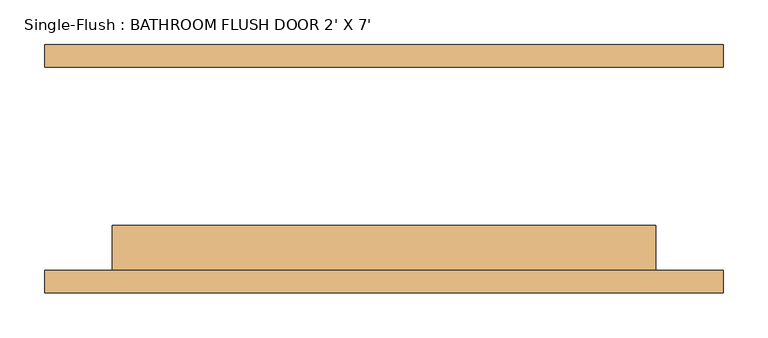
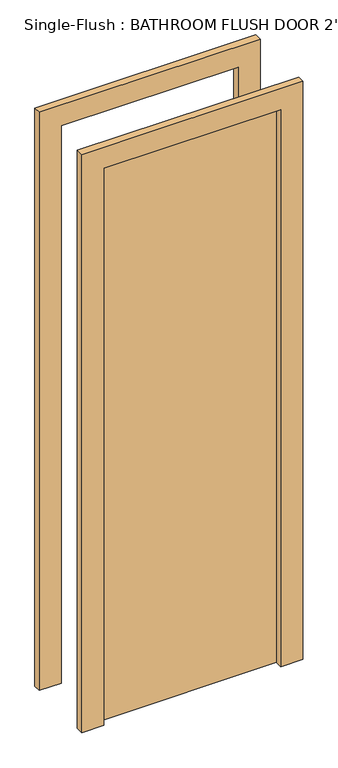
"""IFC4 building model written with IfcOpenShell, lengths in millimetres: door geometry, Single-Flush : BATHROOM FLUSH DOOR 2' X 7'."""

from ifc_helpers import new_model, si_unit, frame, origin, origin_with_axes, place, context, project, spatial, polyline, outline, extrude, source, transform, mapped, element, save


def single_flush_bathroom_flush_door_2_x_7_11f1894d(model_context):
    return source(origin(), model_context, "Body", "SweptSolid", [
        extrude(outline(polyline([(2108.2, -381.0), (0.0, -381.0), (0.0, -304.8), (2032.0, -304.8), (2032.0, 304.8), (0.0, 304.8), (0.0, 381.0), (2108.2, 381.0), (2108.2, -381.0)])), frame((0.0, -139.7, 0.0), z_axis=(0.0, 1.0, 0.0), x_axis=(0.0, 0.0, 1.0)), (0.0, 0.0, 1.0), 25.4),
        extrude(outline(polyline([(2108.2, 381.0), (2108.2, -381.0), (0.0, -381.0), (0.0, -304.8), (2032.0, -304.8), (2032.0, 304.8), (0.0, 304.8), (0.0, 381.0), (2108.2, 381.0)])), frame((0.0, 114.3, 0.0), z_axis=(0.0, 1.0, 0.0), x_axis=(0.0, 0.0, 1.0)), (0.0, 0.0, 1.0), 25.4),
        extrude(outline(polyline([(304.8, -63.5), (304.8, -114.3), (-304.8, -114.3), (-304.8, -63.5), (304.8, -63.5)])), origin_with_axes(), (0.0, 0.0, 1.0), 2032.0),
    ])


if __name__ == "__main__":
    model = new_model("IFC4")
    model_context = context("Model", 3, world=origin())
    ifc_project = project(units=[si_unit("LENGTHUNIT", "METRE", prefix="MILLI")], contexts=[model_context])
    site = spatial("IfcSite", under=ifc_project)
    building = spatial("IfcBuilding", under=site)
    placement = place(None, origin())
    single_flush_bathroom_flush_door_2_x_7_shape = single_flush_bathroom_flush_door_2_x_7_11f1894d(model_context)
    element("IfcDoor", 1, ObjectType="Single-Flush : BATHROOM FLUSH DOOR 2' X 7'", at=placement, inside=building, context=model_context, shape_type="MappedRepresentation", body=[
        mapped(single_flush_bathroom_flush_door_2_x_7_shape, transform((0.0, 0.0, 0.0), x_axis=(1.0, 0.0, 0.0), y_axis=(0.0, 1.0, 0.0), z_axis=(0.0, 0.0, 1.0))),
    ])
    save(model, "model.ifc")

# Revit data of these elements
# Type "Single-Flush : BATHROOM FLUSH DOOR 2' X 7'"
#   Type Mark = "8"
#   Construction Type Id = "MDOOR"
#   Assembly Code = "C1020"
#   Analytic Construction = "Metal"
#   Thickness = 0' - 2"
#   Heat Transfer Coefficient (U) = 0.651978 BTU/(h·ft²·°F)
#   Height = 6' - 8"
#   Trim Projection Ext = 0' - 1"
#   Trim Projection Int = 0' - 1"
#   Trim Width = 0' - 3"
#   Width = 2' - 0"
#   Define Thermal Properties by = 1
#   Door Material = Door - Panel
#   Frame Material = Door - Frame
#   Visual Light Transmittance = 0
#   Solar Heat Gain Coefficient = 0
#   Function = (empty or 0)
#   Wall Closure = (empty or 0)
# Element 1 (IfcDoor, "Single-Flush : BATHROOM FLUSH DOOR 2' X 7'")
#   Materials on its faces: "Door - Frame", "Door - Panel"
# Materials
#   "Door - Panel": class "Wood", colour RGB 210 159 95, transparency 0, Cost = 0
#   "Door - Frame": colour RGB 118 70 51, transparency 0, Cost = 0
